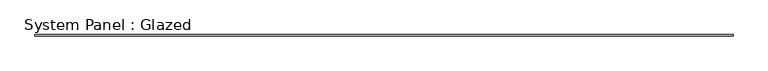
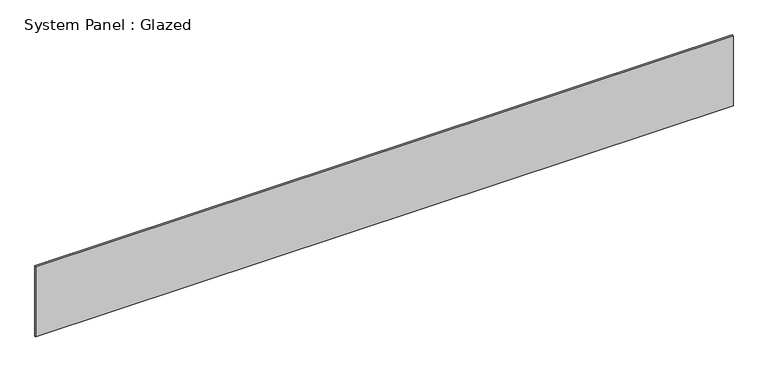
"""IFC4 building model written with IfcOpenShell, lengths in millimetres: plate geometry, System Panel : Glazed."""

from ifc_helpers import new_model, si_unit, origin, origin_with_axes, place, context, project, spatial, polyline, outline, extrude, source, transform, mapped, element, save


def system_panel_glazed_1060ff55(model_context):
    return source(origin(), model_context, "Body", "SweptSolid", [
        extrude(outline(polyline([(6858.0, 19.05), (-6858.0, 19.05), (-6858.0, 44.45), (6858.0, 44.45), (6858.0, 19.05)])), origin_with_axes(), (0.0, 0.0, 1.0), 1460.5),
    ])


if __name__ == "__main__":
    model = new_model("IFC4")
    model_context = context("Model", 3, world=origin())
    ifc_project = project(units=[si_unit("LENGTHUNIT", "METRE", prefix="MILLI")], contexts=[model_context])
    site = spatial("IfcSite", under=ifc_project)
    building = spatial("IfcBuilding", under=site)
    placement = place(None, origin())
    system_panel_glazed_shape = system_panel_glazed_1060ff55(model_context)
    element("IfcPlate", 1, ObjectType="System Panel : Glazed", at=placement, inside=building, context=model_context, shape_type="MappedRepresentation", body=[
        mapped(system_panel_glazed_shape, transform((0.0, 0.0, 0.0), x_axis=(1.0, 0.0, 0.0), y_axis=(0.0, 1.0, 0.0), z_axis=(0.0, 0.0, 1.0))),
    ])
    save(model, "model.ifc")

# Revit data of these elements
# Type "System Panel : Glazed"
#   Construction Type Id = "GSP4R"
#   Analytic Construction = "1/8 in Pilkington single glazing"
#   Visual Light Transmittance = 0.9
#   Solar Heat Gain Coefficient = 0.86
#   Heat Transfer Coefficient (U) = 1.18115 BTU/(h·ft²·°F)
# Element 1 (IfcPlate, "System Panel : Glazed")
#   Materials on its faces: "Glass"
# Materials
#   "Glass": class "Glass", colour RGB 0 128 192, transparency 0.75, Description = "Soda Lime Glass", Cost = 0
